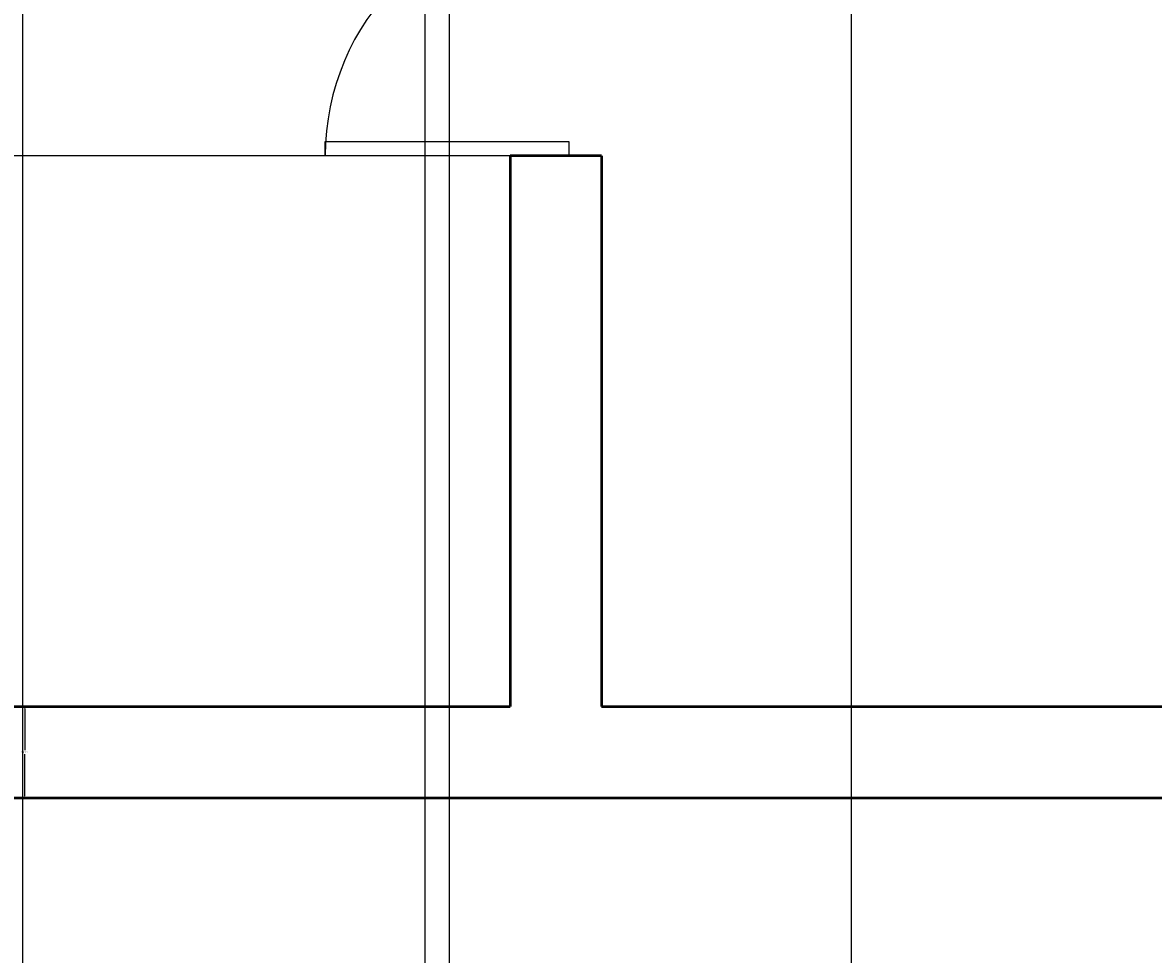
# Model space of a CAD drawing. Units: inches. Extents: x 7359 to 7979, y 33027 to 34263.
# Tile 27 of 32: x 7641 to 7753, y 33749 to 33841. Entities that reach past the tile are written whole.
import ezdxf

# ---------------------------------------------------------------- set-up
doc = ezdxf.new("R2010")
doc.units = ezdxf.units.IN
for name, color, linetype, lineweight in [('A-ANNO-DIMS', 2, 'Continuous', 18), ('A-DOOR', 3, 'Continuous', 25), ('A-WALL', 7, 'Continuous', 50)]:
    doc.layers.add(name, color=color, linetype=linetype, lineweight=lineweight)
doc.styles.get("Standard").update_dxf_attribs({"font": 'arial.ttf'})
doc.dimstyles.get("Standard").update_dxf_attribs({"dimtxt": 0.18, "dimasz": 0.18, "dimexe": 0.18, "dimexo": 0.0625, "dimgap": 0.09, "dimtad": 0, "dimtih": 1, "dimtoh": 1, "dimdec": 4, "dimzin": 0, "dimdsep": 46, "dimtxsty": 'Standard', "dimcen": 0.09, "dimadec": 0, "dimazin": 0, "dimtfac": 1, "dimtdec": 4, "dimtofl": 0, "dimtmove": 0, "dimatfit": 3, "dimfxl": 1, "dimtolj": 1, "dimtzin": 0, "dimarcsym": 0})

# ---------------------------------------------------------------- blocks, each defined once
blk = doc.blocks.new('*U2')
for p, q in [((0, 0), (0, -100)), ((750, 0), (750, -100))]:
    blk.add_line(p, q)
blk.add_lwpolyline([(0, 0), (0, 750), (43.75, 750), (43.75, 0)], close=True)
blk.add_arc((0, 0), 750, 0, 90)
blk = doc.blocks.new('*D63')
at = {"layer": 'A-ANNO-DIMS', "color": 0, "lineweight": -2, "transparency": 16777216}
for p, q in [((7629.94, 33773.83), (7641.88, 33773.83)), ((7641.7, 33773.65), (7641.7, 33769.52)), ((7641.7, 33765.01), (7641.7, 33769.15)), ((7629.94, 33764.83), (7641.88, 33764.83))]:
    blk.add_line(p, q, dxfattribs=at)
at = {"layer": 'A-ANNO-DIMS', "color": 0, "transparency": 16777216}
for points in [[(7641.67, 33773.65), (7641.73, 33773.65), (7641.7, 33773.83)], [(7641.67, 33765.01), (7641.73, 33765.01), (7641.7, 33764.83)]]:
    blk.add_solid(points, dxfattribs=at)
at = {"layer": 'Defpoints', "color": 0, "transparency": 16777216}
for p in [(7629.88, 33773.83), (7641.7, 33773.83), (7629.88, 33764.83)]:
    blk.add_point(p, dxfattribs=at)
at = {"layer": 'A-ANNO-DIMS', "color": 0, "transparency": 16777216, "insert": (7641.7, 33769.33), "char_height": 0.18, "attachment_point": 5}
blk.add_mtext('\\A1;9 TYP.', dxfattribs=at)
blk = doc.blocks.new('*D69')
at = {"layer": 'A-ANNO-DIMS', "color": 0, "lineweight": -2, "transparency": 16777216}
for p, q in [((7681.09, 34081.77), (7681.09, 33632.31)), ((7723.09, 34081.77), (7723.09, 33632.31)), ((7681.27, 33632.49), (7701.87, 33632.49)), ((7722.91, 33632.49), (7702.31, 33632.49))]:
    blk.add_line(p, q, dxfattribs=at)
at = {"layer": 'A-ANNO-DIMS', "color": 0, "transparency": 16777216}
for points in [[(7681.27, 33632.52), (7681.27, 33632.46), (7681.09, 33632.49)], [(7722.91, 33632.52), (7722.91, 33632.46), (7723.09, 33632.49)]]:
    blk.add_solid(points, dxfattribs=at)
at = {"layer": 'Defpoints', "color": 0, "transparency": 16777216}
for p in [(7681.09, 34081.83), (7723.09, 34081.83), (7723.09, 33632.49)]:
    blk.add_point(p, dxfattribs=at)
at = {"layer": 'A-ANNO-DIMS', "color": 0, "transparency": 16777216, "insert": (7702.09, 33632.49), "char_height": 0.18, "attachment_point": 5}
blk.add_mtext('\\A1;42', dxfattribs=at)
blk = doc.blocks.new('*D71')
at = {"layer": 'A-ANNO-DIMS', "color": 0, "lineweight": -2, "transparency": 16777216}
for p, q in [((7641.49, 33907.17), (7641.49, 33632.31)), ((7683.49, 33907.17), (7683.49, 33632.31)), ((7641.67, 33632.49), (7662.27, 33632.49)), ((7683.31, 33632.49), (7662.71, 33632.49))]:
    blk.add_line(p, q, dxfattribs=at)
at = {"layer": 'A-ANNO-DIMS', "color": 0, "transparency": 16777216}
for points in [[(7641.67, 33632.52), (7641.67, 33632.46), (7641.49, 33632.49)], [(7683.31, 33632.52), (7683.31, 33632.46), (7683.49, 33632.49)]]:
    blk.add_solid(points, dxfattribs=at)
at = {"layer": 'Defpoints', "color": 0, "transparency": 16777216}
for p in [(7641.49, 33907.23), (7683.49, 33907.23), (7683.49, 33632.49)]:
    blk.add_point(p, dxfattribs=at)
at = {"layer": 'A-ANNO-DIMS', "color": 0, "transparency": 16777216, "insert": (7662.49, 33632.49), "char_height": 0.18, "attachment_point": 5}
blk.add_mtext('\\A1;42', dxfattribs=at)
blk = doc.blocks.new('*D72')
at = {"layer": 'A-ANNO-DIMS', "color": 0, "lineweight": -2, "transparency": 16777216}
for p, q in [((7689.43, 33876.08), (7359.41, 33876.08)), ((7359.59, 33875.9), (7359.59, 33852.27)), ((7359.59, 33828.26), (7359.59, 33851.9)), ((7689.43, 33828.08), (7359.41, 33828.08))]:
    blk.add_line(p, q, dxfattribs=at)
at = {"layer": 'A-ANNO-DIMS', "color": 0, "transparency": 16777216}
for points in [[(7359.56, 33875.9), (7359.62, 33875.9), (7359.59, 33876.08)], [(7359.56, 33828.26), (7359.62, 33828.26), (7359.59, 33828.08)]]:
    blk.add_solid(points, dxfattribs=at)
at = {"layer": 'Defpoints', "color": 0, "transparency": 16777216}
for p in [(7359.59, 33876.08), (7689.49, 33876.08), (7689.49, 33828.08)]:
    blk.add_point(p, dxfattribs=at)
at = {"layer": 'A-ANNO-DIMS', "color": 0, "transparency": 16777216, "insert": (7359.59, 33852.08), "char_height": 0.18, "attachment_point": 5}
blk.add_mtext('\\A1;48', dxfattribs=at)

msp = doc.modelspace()

# ---------------------------------------------------------------- linework, layer by layer
at = {"layer": 'A-WALL'}
for p, q in [((7698.4915, 33828.0839), (7689.4915, 33828.0839)), ((7689.4915, 33828.0839), (7689.4915, 33773.8339)), ((7698.4915, 33828.0839), (7698.4915, 33773.8339)), ((7467.5915, 33773.8339), (7689.4915, 33773.8339)), ((7698.4915, 33773.8339), (7874.9915, 33773.8339)), ((7458.5915, 33764.8339), (7883.9915, 33764.8339))]:
    msp.add_line(p, q, dxfattribs=at)

# ---------------------------------------------------------------- block references
at = {"layer": 'A-DOOR', "xscale": 0.0319999999999999, "yscale": 0.0319999999999999, "zscale": 0.0319999999999999, "rotation": 90}
msp.add_blockref('*U2', (7695.2915, 33828.0839), dxfattribs=at)

# ---------------------------------------------------------------- dimensions: what is measured, and where the dimension line sits
at = {"layer": 'A-ANNO-DIMS'}
for base, p1, p2, picture, middle in [((7723.0915, 33632.4891), (7681.0915, 34081.8339), (7723.0915, 34081.8339), '*D69', (7702.0915, 33632.4891)), ((7683.4915, 33632.4891), (7641.4915, 33907.2339), (7683.4915, 33907.2339), '*D71', (7662.4915, 33632.4891))]:
    dim = msp.add_linear_dim(base=base, p1=p1, p2=p2, dimstyle='Standard', override={"dimdec": 0, "dimlfac": 1, "dimrnd": 0, "dimzin": 0, "dimdsep": 46, "dimlunit": 2}, dxfattribs=at)
    dim.commit()
    dim.dimension.update_dxf_attribs({"geometry": picture, "text_midpoint": middle})
dim = msp.add_linear_dim(base=(7359.5866, 33876.0839), p1=(7689.4915, 33828.0839), p2=(7689.4915, 33876.0839), angle=90, dimstyle='Standard', override={"dimdec": 0, "dimlfac": 1, "dimrnd": 0, "dimzin": 0, "dimdsep": 46, "dimlunit": 2}, dxfattribs=at)
dim.commit()
dim.dimension.update_dxf_attribs({"geometry": '*D72', "text_midpoint": (7359.5866, 33852.0839)})
dim = msp.add_linear_dim(base=(7641.6969, 33773.8339), p1=(7629.8778, 33764.8339), p2=(7629.8778, 33773.8339), angle=90, text='<> TYP.', dimstyle='Standard', override={"dimdec": 0, "dimlfac": 1, "dimrnd": 0, "dimzin": 0, "dimdsep": 46, "dimlunit": 2}, dxfattribs=at)
dim.commit()
dim.dimension.update_dxf_attribs({"geometry": '*D63', "text_midpoint": (7641.6969, 33769.3339)})

doc.saveas('drawing.dxf')
